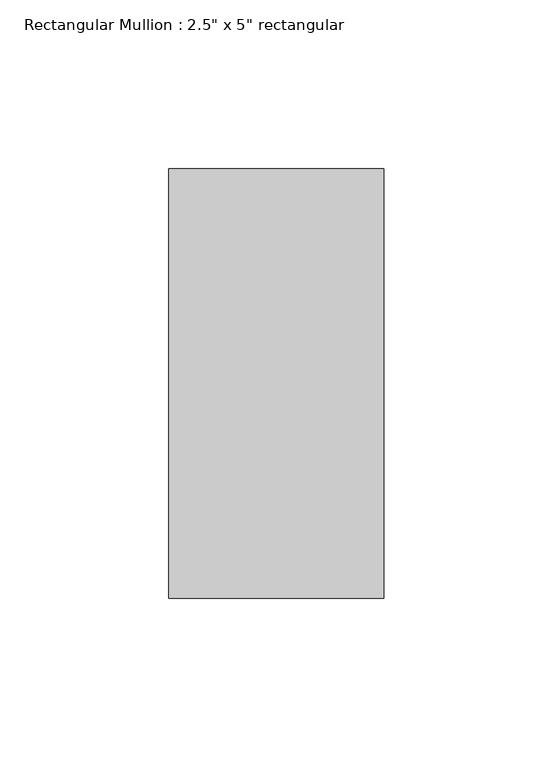
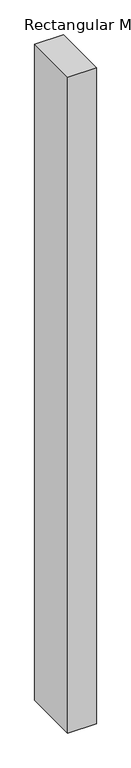
"""IFC4 building model written with IfcOpenShell, lengths in millimetres: member geometry."""

from ifc_helpers import new_model, si_unit, frame, origin, place, context, project, spatial, polyline, outline, extrude, source, transform, mapped, element, save


def member_811bfb9a(model_context):
    return source(origin(), model_context, "Body", "SweptSolid", [
        extrude(outline(polyline([(0.0, 63.5), (0.0, -63.5), (-63.5, -63.5), (-63.5, 63.5), (0.0, 63.5)])), frame((0.0, 0.0, -1539.2746189), z_axis=(0.0, 0.0, 1.0), x_axis=(1.0, 0.0, 0.0)), (0.0, 0.0, 1.0), 1539.2746189),
    ])


if __name__ == "__main__":
    model = new_model("IFC4")
    model_context = context("Model", 3, world=origin())
    ifc_project = project(units=[si_unit("LENGTHUNIT", "METRE", prefix="MILLI")], contexts=[model_context])
    site = spatial("IfcSite", under=ifc_project)
    building = spatial("IfcBuilding", under=site)
    placement = place(None, origin())
    member_shape = member_811bfb9a(model_context)
    element("IfcMember", 1, ObjectType="Rectangular Mullion : 2.5\" x 5\" rectangular", at=placement, inside=building, context=model_context, shape_type="MappedRepresentation", body=[
        mapped(member_shape, transform((0.0, 0.0, 0.0), x_axis=(1.0, 0.0, 0.0), y_axis=(0.0, 1.0, 0.0), z_axis=(0.0, 0.0, 1.0))),
    ])
    save(model, "model.ifc")

# Revit data of these elements
# Type "Rectangular Mullion : 2.5\" x 5\" rectangular"
#   built-in parameter 1007304 = 0.416667 (stored number, unit not read)
#   built-in parameter 1007301 = 0.104167 (stored number, unit not read)
#   built-in parameter 1007300 = 0.104167 (stored number, unit not read)
# Element 1 (IfcMember, "Rectangular Mullion : 2.5\" x 5\" rectangular")
#   Materials on its faces: "Aluminum"
# Materials
#   "Aluminum": class "Metal", colour RGB 247 247 247, transparency 0, Description = "Aluminum 6061", Cost = 0
